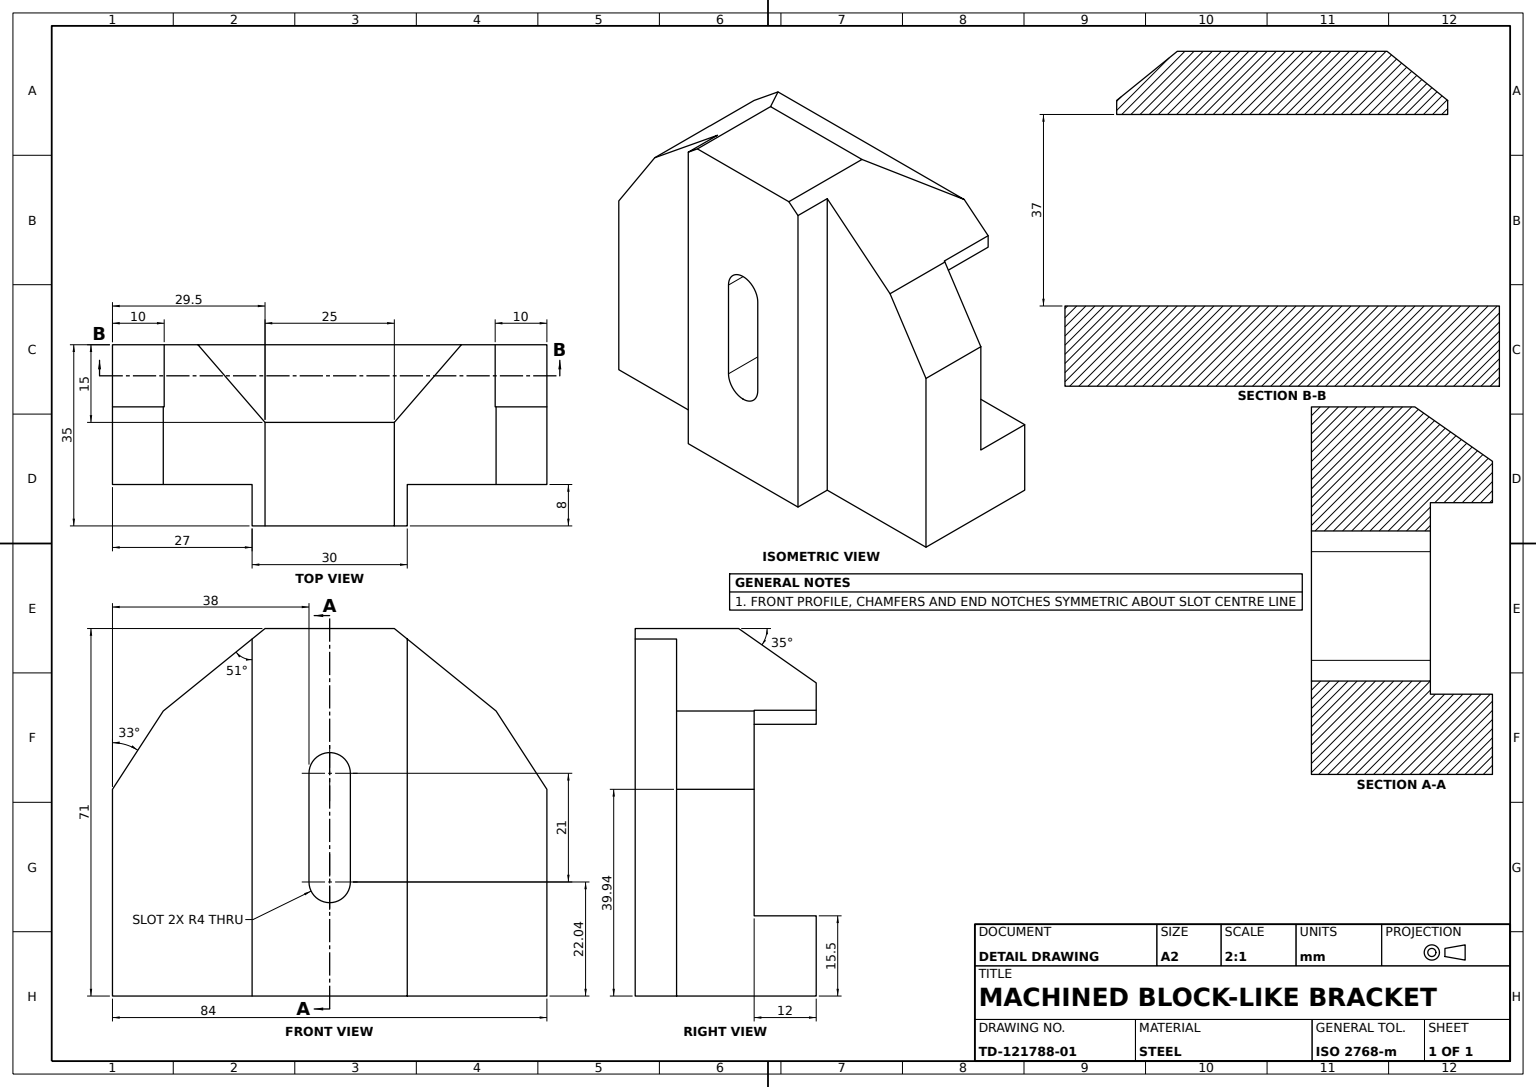
from build123d import *

# Parameters (mm, degrees)
BASE_BLOCK_84MM_DEPTH  = 84
BACK_CHANNEL_SKETCH_W  = 12
BACK_CHANNEL_SKETCH_H  = 10
BACK_CHANNEL_CUT_DEPTH = 84
FRONT_PAD_SKETCH_W     = 8
FRONT_PAD_SKETCH_H     = 71
FRONT_PAD_8MM_DEPTH    = 15
TOP_CHAMFER_CUT_DEPTH  = 42.5
SLOT_CUT_DEPTH         = 75


with BuildPart() as part:
    # Block Profile Sketch → Base Block 84mm (new body)
    with BuildSketch(Plane.XY):
        Polygon((0, 0), (27, 0), (27, 71), (15, 71), (0, 60.496886927), (0, 52.496886927), (12, 52.496886927), (12, 15.496886927), (0, 15.496886927), align=None)
    extrude(amount=BASE_BLOCK_84MM_DEPTH)

    # Back Channel Sketch → Back Channel Cut (cut)
    with BuildSketch(Plane(origin=(0, 15.496886927, 0), x_dir=(1, 0, 0), z_dir=(0, 1, 0))):
        with Locations((6, -79)):
            Rectangle(BACK_CHANNEL_SKETCH_W, BACK_CHANNEL_SKETCH_H)
        with Locations((6, -5)):
            Rectangle(BACK_CHANNEL_SKETCH_W, BACK_CHANNEL_SKETCH_H)
    extrude(amount=BACK_CHANNEL_CUT_DEPTH, mode=Mode.SUBTRACT)

    # Front Pad Sketch → Front Pad 8mm (add, symmetric)
    with BuildSketch(Plane.XY.offset(42)):
        with Locations((31, 35.5)):
            Rectangle(FRONT_PAD_SKETCH_W, FRONT_PAD_SKETCH_H)
    extrude(amount=FRONT_PAD_8MM_DEPTH, both=True)

    # Top Chamfer Sketch → Top Chamfer Cut (cut, symmetric)
    with BuildSketch(Plane(origin=(27, 0, 0), x_dir=(0, 0, -1), z_dir=(1, 0, 0))):
        Polygon((-54.5, 71), (-74.175600087, 55.067013206), (-84, 39.938763989), (-84, 71), align=None)
        Polygon((-29.5, 71), (-9.824399913, 55.067013206), (0, 39.938763989), (0, 71), align=None)
    extrude(amount=TOP_CHAMFER_CUT_DEPTH, both=True, mode=Mode.SUBTRACT)

    # Slot Sketch → Slot Cut (cut)
    with BuildSketch(Plane.ZY.offset(-12)):
        with BuildLine():
            Line((46, 43.035553087), (46, 22.035553087))
            ThreePointArc((46, 22.035553087), (42, 18.035553087), (38, 22.035553087))
            Line((38, 22.035553087), (38, 43.035553087))
            ThreePointArc((38, 43.035553087), (42, 47.035553087), (46, 43.035553087))
        make_face()
    extrude(amount=-SLOT_CUT_DEPTH, mode=Mode.SUBTRACT)


solid = part.part
